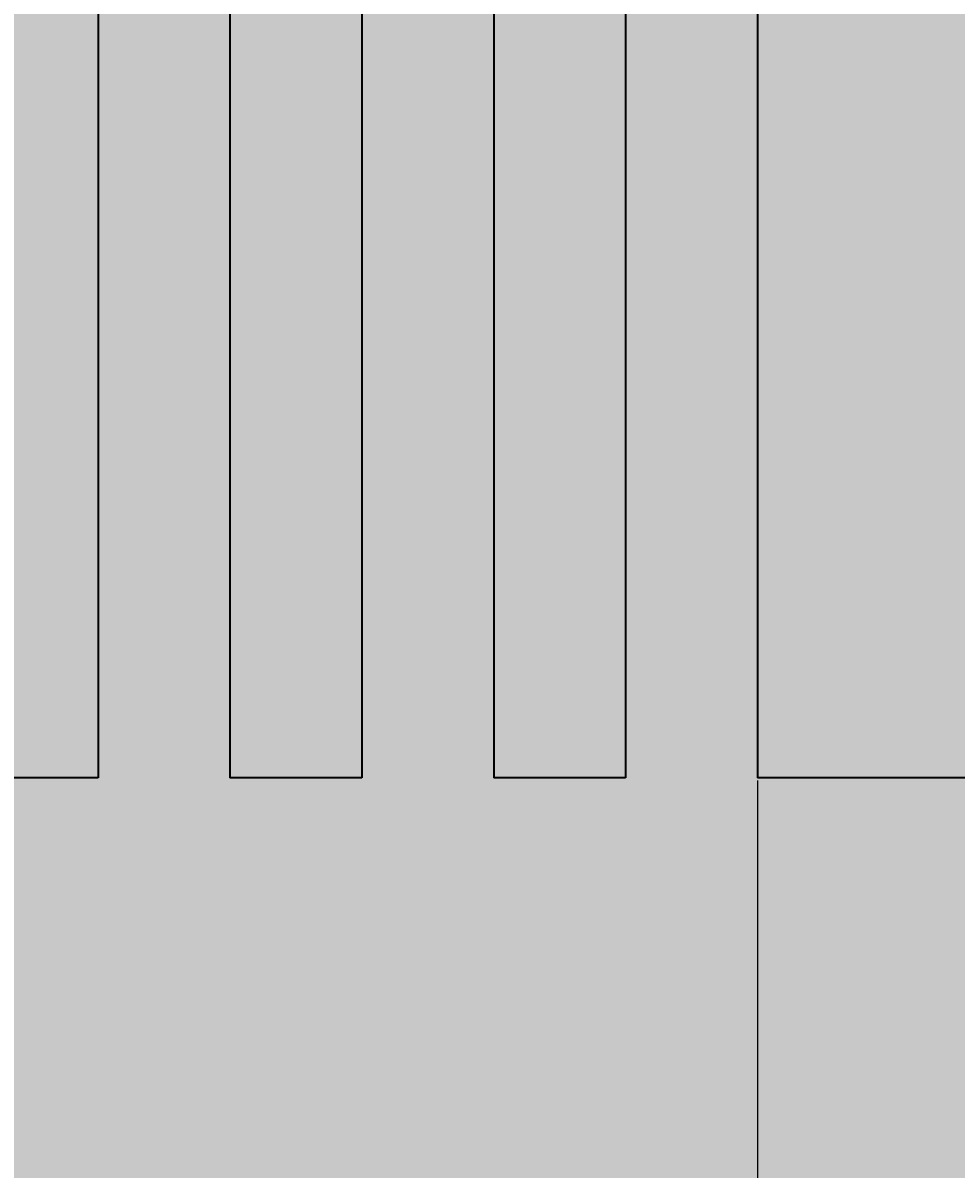
# Model space of a CAD drawing. Units: inches. Extents: x -1 to 292, y -3 to 199.
# Tile 23 of 52: x 106 to 127, y 42 to 68. Entities that reach past the tile are written whole.
import ezdxf

# ---------------------------------------------------------------- set-up
doc = ezdxf.new("R2010")
doc.units = ezdxf.units.IN
doc.header["$MEASUREMENT"] = 0
for name, color, linetype, lineweight in [('M-DIMS', 2, 'Continuous', 18), ('M-EQPM', 7, 'Continuous', 35), ('M-PATT', 8, 'Continuous', 13)]:
    doc.layers.add(name, color=color, linetype=linetype, lineweight=lineweight)
doc.styles.get("Standard").update_dxf_attribs({"font": 'arial.ttf'})
doc.dimstyles.get("Standard").update_dxf_attribs({"dimtxt": 0.18, "dimasz": 0.18, "dimexe": 0.18, "dimexo": 0.0625, "dimgap": 0.09, "dimtad": 0, "dimtih": 1, "dimtoh": 1, "dimdec": 4, "dimzin": 0, "dimdsep": 46, "dimtxsty": 'Standard', "dimcen": 0.09, "dimadec": 0, "dimazin": 0, "dimtfac": 1, "dimtdec": 4, "dimtofl": 0, "dimtmove": 0, "dimatfit": 3, "dimfxl": 1, "dimtolj": 1, "dimtzin": 0, "dimarcsym": 0})

# ---------------------------------------------------------------- blocks, each defined once
blk = doc.blocks.new('BOILER-TUBE')
for p, q in [((0, 40.63), (0, 0)), ((3, 40.63), (3, 0))]:
    blk.add_line(p, q)
blk.add_lwpolyline([(3, 0), (0, 0)])
blk = doc.blocks.new('*D7')
at = {"layer": 'Defpoints', "color": 0, "transparency": 16777216}
for p in [(21.861, 54.582), (205.115, 54.582), (21.861, 39.982)]:
    blk.add_point(p, dxfattribs=at)
at = {"layer": 'M-DIMS', "color": 0, "lineweight": -2, "transparency": 16777216}
for p, q in [((21.861, 54.52), (21.861, 39.802)), ((205.115, 54.52), (205.115, 39.802)), ((22.041, 39.982), (113.033, 39.982)), ((204.935, 39.982), (113.944, 39.982))]:
    blk.add_line(p, q, dxfattribs=at)
at = {"layer": 'M-DIMS', "color": 0, "transparency": 16777216}
for points in [[(22.041, 40.012), (22.041, 39.952), (21.861, 39.982)], [(204.935, 40.012), (204.935, 39.952), (205.115, 39.982)]]:
    blk.add_solid(points, dxfattribs=at)
at = {"layer": 'M-DIMS', "color": 0, "transparency": 16777216, "insert": (113.488, 39.982), "char_height": 0.18, "attachment_point": 5}
blk.add_mtext('\\A1;183.25', dxfattribs=at)
blk = doc.blocks.new('*D8')
at = {"layer": 'Defpoints', "color": 0, "transparency": 16777216}
for p in [(-0.662, 126.765), (111.488, 126.765), (69.013, 25.514)]:
    blk.add_point(p, dxfattribs=at)
at = {"layer": 'M-DIMS', "color": 0, "lineweight": -2, "transparency": 16777216}
for p, q in [((111.426, 126.765), (-0.842, 126.765)), ((-0.662, 126.585), (-0.662, 76.321)), ((-0.662, 25.694), (-0.662, 75.958)), ((68.951, 25.514), (-0.842, 25.514))]:
    blk.add_line(p, q, dxfattribs=at)
at = {"layer": 'M-DIMS', "color": 0, "transparency": 16777216}
for points in [[(-0.692, 126.585), (-0.632, 126.585), (-0.662, 126.765)], [(-0.692, 25.694), (-0.632, 25.694), (-0.662, 25.514)]]:
    blk.add_solid(points, dxfattribs=at)
at = {"layer": 'M-DIMS', "color": 0, "transparency": 16777216, "insert": (-0.662, 76.14), "char_height": 0.18, "attachment_point": 5}
blk.add_mtext('\\A1;101.25', dxfattribs=at)
blk = doc.blocks.new('*D22')
at = {"layer": 'Defpoints', "color": 0, "transparency": 16777216}
for p in [(82.679, 51.267), (122.679, 51.267), (122.679, -2.71)]:
    blk.add_point(p, dxfattribs=at)
at = {"layer": 'M-DIMS', "color": 0, "lineweight": -2, "transparency": 16777216}
for p, q in [((82.679, 51.205), (82.679, -2.89)), ((122.679, 51.205), (122.679, -2.89)), ((82.859, -2.71), (102.457, -2.71)), ((122.499, -2.71), (102.901, -2.71))]:
    blk.add_line(p, q, dxfattribs=at)
at = {"layer": 'M-DIMS', "color": 0, "transparency": 16777216}
for points in [[(82.859, -2.68), (82.859, -2.74), (82.679, -2.71)], [(122.499, -2.68), (122.499, -2.74), (122.679, -2.71)]]:
    blk.add_solid(points, dxfattribs=at)
at = {"layer": 'M-DIMS', "color": 0, "transparency": 16777216, "insert": (102.679, -2.71), "char_height": 0.18, "attachment_point": 5}
blk.add_mtext('\\A1;40', dxfattribs=at)

msp = doc.modelspace()

# ---------------------------------------------------------------- hatches: boundary and pattern name
at = {"layer": 'M-PATT'}
h = msp.add_hatch(color=256, dxfattribs=at)
h.set_gradient(color1=(237, 31, 36), color2=(242, 113, 114), tint=1, name='CYLINDER')
h.paths.add_polyline_path([(106.0735, 105.9941), (106.0735, 106.9941), (108.0603, 106.9941), (107.8488, 107.6501), (57.8007, 107.6501, 0.4142136), (49.9241, 99.7735), (52.3176, 101.3278), (55.0097, 99.7735), (57.4032, 101.3278), (60.0953, 99.7735), (62.4888, 101.3278), (65.1809, 99.7735), (67.5744, 101.3278), (70.2665, 99.7735), (72.66, 101.3278), (75.3521, 99.7735), (77.7456, 101.3278), (80.4377, 99.7735), (82.8312, 101.3278), (85.5233, 99.7735), (87.9168, 101.3278), (90.6089, 99.7735), (93.0024, 101.3278), (95.6945, 99.7735), (98.088, 101.3278), (100.7801, 99.7735), (103.1736, 101.3278), (105.8657, 99.7735), (108.2592, 101.3278), (110.9513, 99.7735), (113.3448, 101.3278), (116.0369, 99.7735), (118.4304, 101.3278), (121.1225, 99.7735), (123.516, 101.3278), (126.2082, 99.7735), (128.6016, 101.3278), (131.2938, 99.7735), (133.6872, 101.3278), (136.3794, 99.7735), (138.7728, 101.3278), (141.465, 99.7735), (143.8584, 101.3278), (146.5506, 99.7735), (148.944, 101.3278), (151.6362, 99.7735), (154.0296, 101.3278), (156.7218, 99.7735), (159.1152, 101.3278), (160.6222, 100.4578), (160.6222, 107.6501), (115.4883, 107.6501), (115.4883, 106.9941), (120.9032, 106.9941), (120.9032, 105.9941), (120.9032, 103.3981), (106.0735, 103.3981)])
h.paths.add_polyline_path([(169.176, 107.6501), (162.1623, 107.6501), (162.1623, 100.004), (164.2008, 101.3278), (166.893, 99.7735), (169.2864, 101.3278), (171.9786, 99.7735), (174.372, 101.3278), (177.0526, 99.7802, 0.4139642)])
h.paths.add_polyline_path([(111.4883, 107.6501), (107.8488, 107.6501), (108.0603, 106.9941), (111.4883, 106.9941)], flags=17)
h.paths.add_polyline_path([(61.6788, 91.897), (57.8007, 91.897, -0.1099266), (54.4604, 92.6403), (43.2011, 92.6403), (23.9502, 84.4688), (23.9502, 58.376), (43.2011, 47.2615), (50.9409, 47.2615, -0.2705926), (57.8007, 51.2672), (61.6788, 51.2672)])
h.paths.add_polyline_path([(73.6788, 91.897), (70.6788, 91.897), (70.6788, 51.2672), (73.6788, 51.2672)])
h.paths.add_polyline_path([(79.6788, 91.897), (76.6788, 91.897), (76.6788, 51.2672), (79.6788, 51.2672)])
h.paths.add_polyline_path([(67.6788, 91.897), (64.6788, 91.897), (64.6788, 51.2672), (67.6788, 51.2672)])
h.paths.add_polyline_path([(101.6788, 91.897), (82.6788, 91.897), (82.6788, 51.2672), (101.6788, 51.2672)])
h.paths.add_polyline_path([(107.6788, 91.897), (104.6788, 91.897), (104.6788, 51.2672), (107.6788, 51.2672)])
h.paths.add_polyline_path([(113.6788, 91.897), (110.6788, 91.897), (110.6788, 51.2672), (113.6788, 51.2672)])
h.paths.add_polyline_path([(119.6788, 91.897), (116.6788, 91.897), (116.6788, 51.2672), (119.6788, 51.2672)])
h.paths.add_polyline_path([(141.6788, 91.897), (122.6788, 91.897), (122.6788, 51.2672), (141.6788, 51.2672)])
h.paths.add_polyline_path([(147.6788, 91.897), (144.6788, 91.897), (144.6788, 51.2672), (147.6788, 51.2672)])
h.paths.add_polyline_path([(153.6788, 91.897), (150.6788, 91.897), (150.6788, 51.2672), (153.6788, 51.2672)])
h.paths.add_polyline_path([(159.6788, 91.897), (156.6788, 91.897), (156.6788, 51.2672), (159.6788, 51.2672)])
h.paths.add_polyline_path([(179.5897, 92.6403), (172.5163, 92.6403, -0.1099266), (169.176, 91.897), (162.6788, 91.897), (162.6788, 51.2672), (169.176, 51.2672, -0.2705926), (176.0358, 47.2615), (179.5897, 47.2615)])
h.paths.add_polyline_path([(203.0265, 84.4688), (183.7755, 92.6403), (181.5897, 92.6403), (181.5897, 47.2615), (183.7755, 47.2615), (203.0265, 58.376)])
h.paths.add_polyline_path([(184.4188, 61.52), (200.7224, 61.52), (200.7224, 77.7532), (184.4188, 77.7532)], flags=24)
h = msp.add_hatch(color=256, dxfattribs=at)
h.set_gradient(color1=(0, 255, 255), color2=(0, 255, 255), tint=1)
h.paths.add_polyline_path([(75.3521, 99.7735), (72.66, 101.3278), (70.2665, 99.7735), (67.5744, 101.3278), (65.1809, 99.7735), (62.4888, 101.3278), (60.0953, 99.7735), (57.4032, 101.3278), (55.0097, 99.7735), (52.3176, 101.3278), (49.9241, 99.7735, 0.4142136), (57.8007, 91.897), (61.6788, 91.897), (61.6788, 51.2672), (57.8007, 51.2672, 0.8088808), (54.5813, 36.2021), (65.0947, 51.2672), (64.6788, 51.2672), (64.6788, 91.897), (67.6788, 91.897), (67.6788, 51.2672), (65.0947, 51.2672), (54.5813, 36.2021, 0.1056561), (57.8007, 35.5141), (169.176, 35.5141, 1), (169.176, 51.2672), (162.6788, 51.2672), (162.6788, 91.897), (169.176, 91.897, 0.4144629), (177.0526, 99.7802), (174.372, 101.3278), (171.9786, 99.7735), (169.2864, 101.3278), (166.893, 99.7735), (164.2008, 101.3278), (162.1623, 100.004), (162.1623, 96.1027), (160.6222, 96.1027), (160.6222, 100.4578), (159.1152, 101.3278), (156.7218, 99.7735), (154.0296, 101.3278), (151.6362, 99.7735), (148.944, 101.3278), (146.5506, 99.7735), (143.8584, 101.3278), (141.465, 99.7735), (138.7728, 101.3278), (136.3794, 99.7735), (133.6872, 101.3278), (131.2938, 99.7735), (128.6016, 101.3278), (126.2082, 99.7735), (123.516, 101.3278), (121.1225, 99.7735), (118.4304, 101.3278), (116.0369, 99.7735), (113.3448, 101.3278), (110.9513, 99.7735), (108.2592, 101.3278), (105.8657, 99.7735), (103.1736, 101.3278), (100.7801, 99.7735), (98.088, 101.3278), (95.6945, 99.7735), (93.0024, 101.3278), (90.6089, 99.7735), (87.9168, 101.3278), (85.5233, 99.7735), (82.8312, 101.3278), (80.4377, 99.7735), (77.7456, 101.3278)])
h.paths.add_polyline_path([(79.6788, 91.897), (79.6788, 51.2672), (76.6788, 51.2672), (76.6788, 91.897)], flags=16)
h.paths.add_polyline_path([(73.6788, 91.897), (73.6788, 51.2672), (70.6788, 51.2672), (70.6788, 91.897)], flags=16)
h.paths.add_polyline_path([(82.6788, 91.897), (101.6788, 91.897), (101.6788, 51.2672), (82.6788, 51.2672)], flags=16)
h.paths.add_polyline_path([(104.6788, 91.897), (107.6788, 91.897), (107.6788, 51.2672), (104.6788, 51.2672)], flags=16)
h.paths.add_polyline_path([(110.6788, 91.897), (113.6788, 91.897), (113.6788, 51.2672), (110.6788, 51.2672)], flags=16)
h.paths.add_polyline_path([(116.6788, 91.897), (119.6788, 91.897), (119.6788, 51.2672), (116.6788, 51.2672)], flags=16)
h.paths.add_polyline_path([(122.6788, 91.897), (141.6788, 91.897), (141.6788, 51.2672), (144.6788, 51.2672), (144.6788, 91.897), (147.6788, 91.897), (147.6788, 51.2672), (122.6788, 51.2672)], flags=16)
h.paths.add_polyline_path([(150.6788, 91.897), (153.6788, 91.897), (153.6788, 51.2672), (150.6788, 51.2672)], flags=16)
h.paths.add_polyline_path([(156.6788, 91.897), (159.6788, 91.897), (159.6788, 51.2672), (156.6788, 51.2672)], flags=16)

# ---------------------------------------------------------------- linework, layer by layer
at = {"layer": 'M-EQPM'}
msp.add_line((122.6788, 91.897), (122.6788, 51.2672), dxfattribs=at)
msp.add_lwpolyline([(147.6788, 51.2672), (122.6788, 51.2672)], dxfattribs=at)

# ---------------------------------------------------------------- block references
for p in [(104.679, 51.267), (110.679, 51.267), (116.679, 51.267)]:
    msp.add_blockref('BOILER-TUBE', p, dxfattribs=at)

# ---------------------------------------------------------------- dimensions: what is measured, and where the dimension line sits
at = {"layer": 'M-DIMS'}
for base, p1, p2, angle, picture, middle in [((-0.6625, 126.765), (69.013, 25.5141), (111.4883, 126.765), 90, '*D8', (-0.6625, 76.1396)), ((21.8612, 39.9821), (205.1155, 54.5821), (21.8612, 54.5821), 180, '*D7', (113.4883, 39.9821))]:
    dim = msp.add_linear_dim(base=base, p1=p1, p2=p2, angle=angle, dimstyle='Standard', override={"dimdec": 2, "dimlfac": 1, "dimrnd": 0, "dimzin": 0, "dimdsep": 46, "dimlunit": 2}, dxfattribs=at)
    dim.commit()
    dim.dimension.update_dxf_attribs({"geometry": picture, "text_midpoint": middle})
dim = msp.add_linear_dim(base=(122.6788, -2.7104), p1=(82.6788, 51.2672), p2=(122.6788, 51.2672), dimstyle='Standard', override={"dimdec": 0, "dimlfac": 1, "dimrnd": 0, "dimzin": 0, "dimdsep": 46, "dimlunit": 2}, dxfattribs=at)
dim.commit()
dim.dimension.update_dxf_attribs({"geometry": '*D22', "text_midpoint": (102.6788, -2.7104)})

doc.saveas('drawing.dxf')
